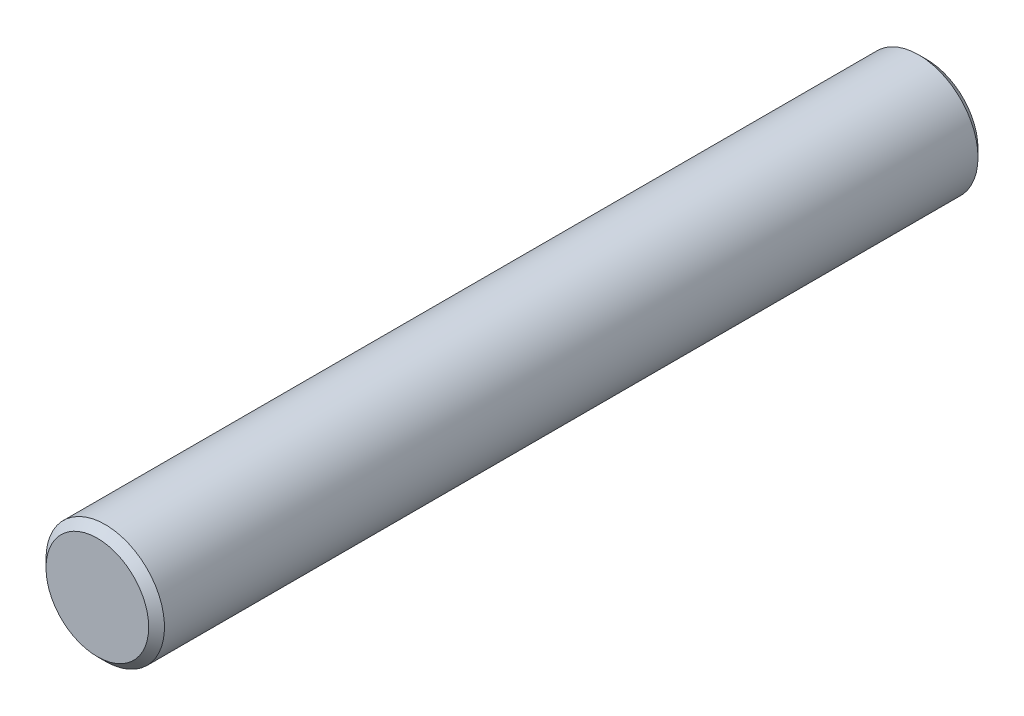
from build123d import *

# Parameters (mm, degrees)
PIN_PROFILE_3_R          = 1.5
PIN_BODY_3X21_DEPTH      = 10.5
END_CHAMFERS_0_2X45_SIZE = 0.2


with BuildPart() as part:
    # Pin Profile Ø3 → Pin Body Ø3x21 (new, symmetric)
    with BuildSketch(Plane.XY):
        with Locations(Location((0, 0, 0), (0, 0, 180))):
            Circle(PIN_PROFILE_3_R)
    extrude(amount=PIN_BODY_3X21_DEPTH, both=True)

    # End Chamfers 0.2x45°
    end_chamfers_0_2x45_edges = [part.edges().sort_by_distance(p)[0] for p in [
        (1.5, 0, -10.5),
        (1.5, 0, 10.5),
    ]]
    chamfer(end_chamfers_0_2x45_edges, length=END_CHAMFERS_0_2X45_SIZE)


solid = part.part
